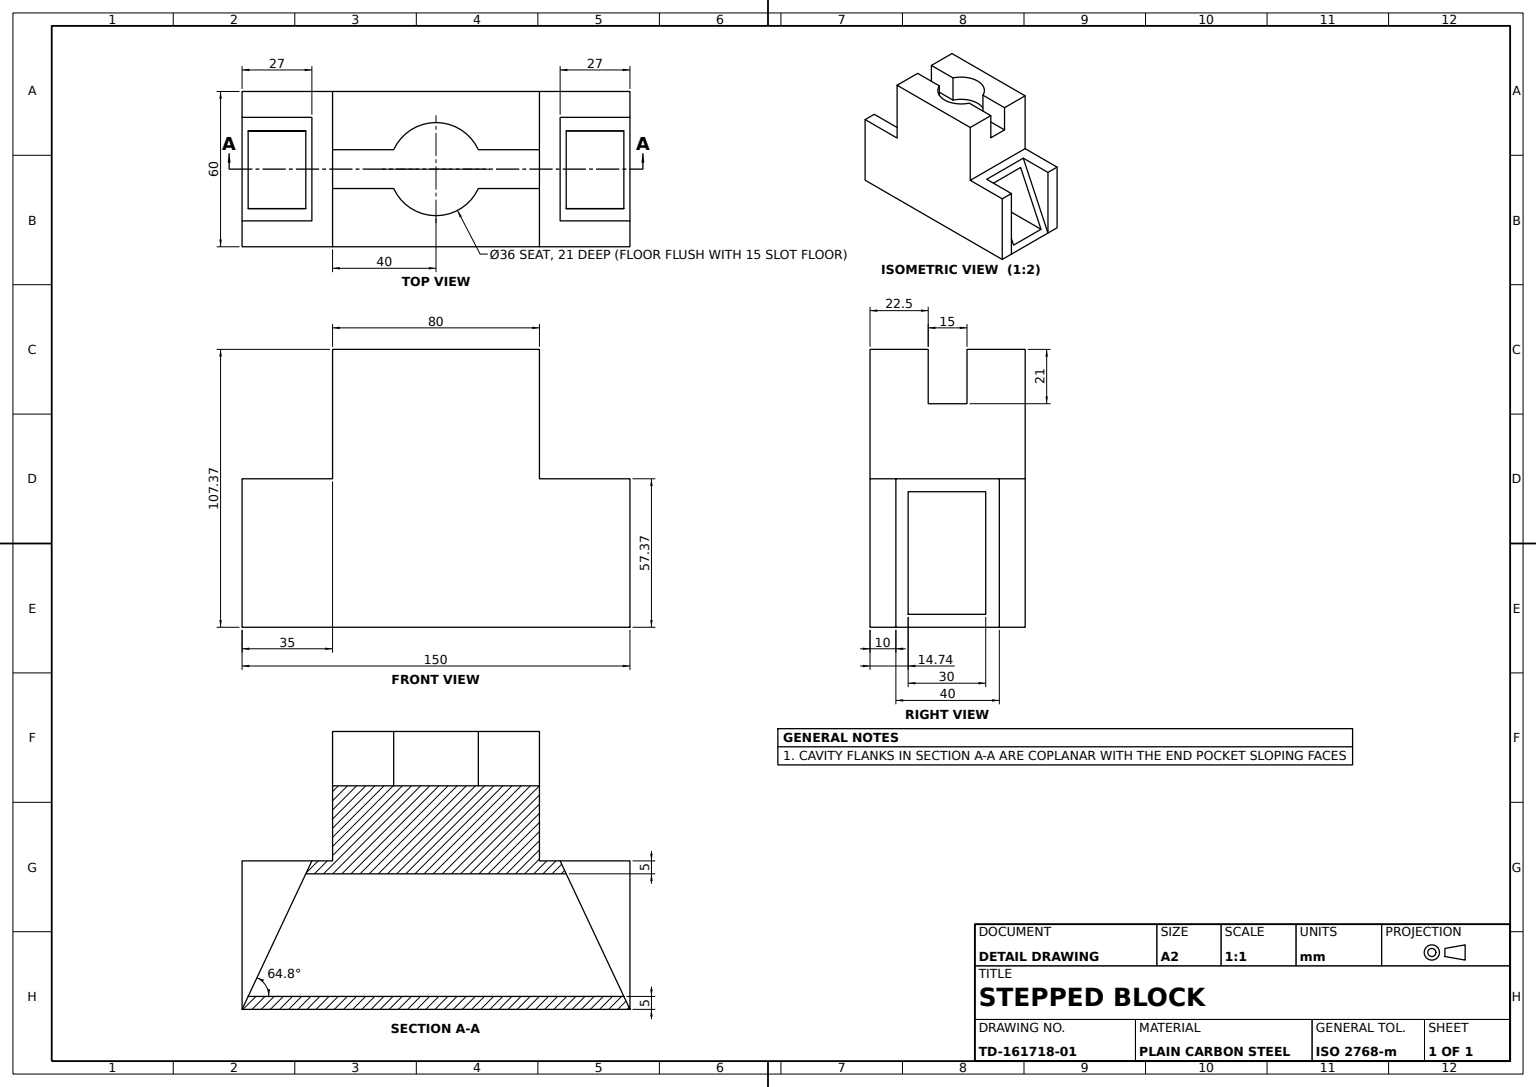
from build123d import *

# Parameters (mm, degrees)
BASE_BLOCK_DEPTH              = 60
TOP_SLOT_WITH_BORE_SEAT_DEPTH = 21
END_CHANNEL_PROFILE_W         = 30
END_CHANNEL_PROFILE_H         = 47.374117648
END_CHANNEL_CUT_DEPTH         = 180.69878471
TRIANGULAR_POCKET_CUT_DEPTH   = 40


with BuildPart() as part:
    # Base Block Profile → Base Block (new body)
    with BuildSketch(Plane.XY):
        Polygon((40, 28.687058824), (75, 28.687058824), (75, -28.687058824), (-75, -28.687058824), (-75, 28.687058824), (-40, 28.687058824), (-40, 78.687058824), (40, 78.687058824), align=None)
    extrude(amount=-BASE_BLOCK_DEPTH)

    # Top Slot Profile → Top Slot With Bore Seat (cut)
    with BuildSketch(Plane(origin=(0, 78.687058824, 0), x_dir=(1, 0, 0), z_dir=(0, 1, 0))):
        with BuildLine():
            Line((-40, 37.5), (-16.363068172, 37.5))
            ThreePointArc((-16.363068172, 37.5), (0, 48), (16.363068172, 37.5))
            Line((16.363068172, 37.5), (40, 37.5))
            Line((40, 37.5), (40, 22.5))
            Line((40, 22.5), (16.363068172, 22.5))
            ThreePointArc((16.363068172, 22.5), (0, 12), (-16.363068172, 22.5))
            Line((-16.363068172, 22.5), (-40, 22.5))
            Line((-40, 22.5), (-40, 37.5))
        make_face()
    extrude(amount=-TOP_SLOT_WITH_BORE_SEAT_DEPTH, mode=Mode.SUBTRACT)

    # End Channel Profile → End Channel Cut (cut, through all)
    with BuildSketch(Plane.ZY.offset(75)):
        with Locations((-29.740602956, 0)):
            Rectangle(END_CHANNEL_PROFILE_W, END_CHANNEL_PROFILE_H)
    extrude(amount=-END_CHANNEL_CUT_DEPTH, mode=Mode.SUBTRACT)

    # Triangular Pocket Profile → Triangular Pocket Cut (cut)
    with BuildSketch(Plane.XY.offset(-10)):
        Polygon((-48, 28.687058824), (-75, -28.687058824), (-75, 28.687058824), align=None)
        Polygon((48, 28.687058824), (75, -28.687058824), (75, 28.687058824), align=None)
    extrude(amount=-TRIANGULAR_POCKET_CUT_DEPTH, mode=Mode.SUBTRACT)


solid = part.part
